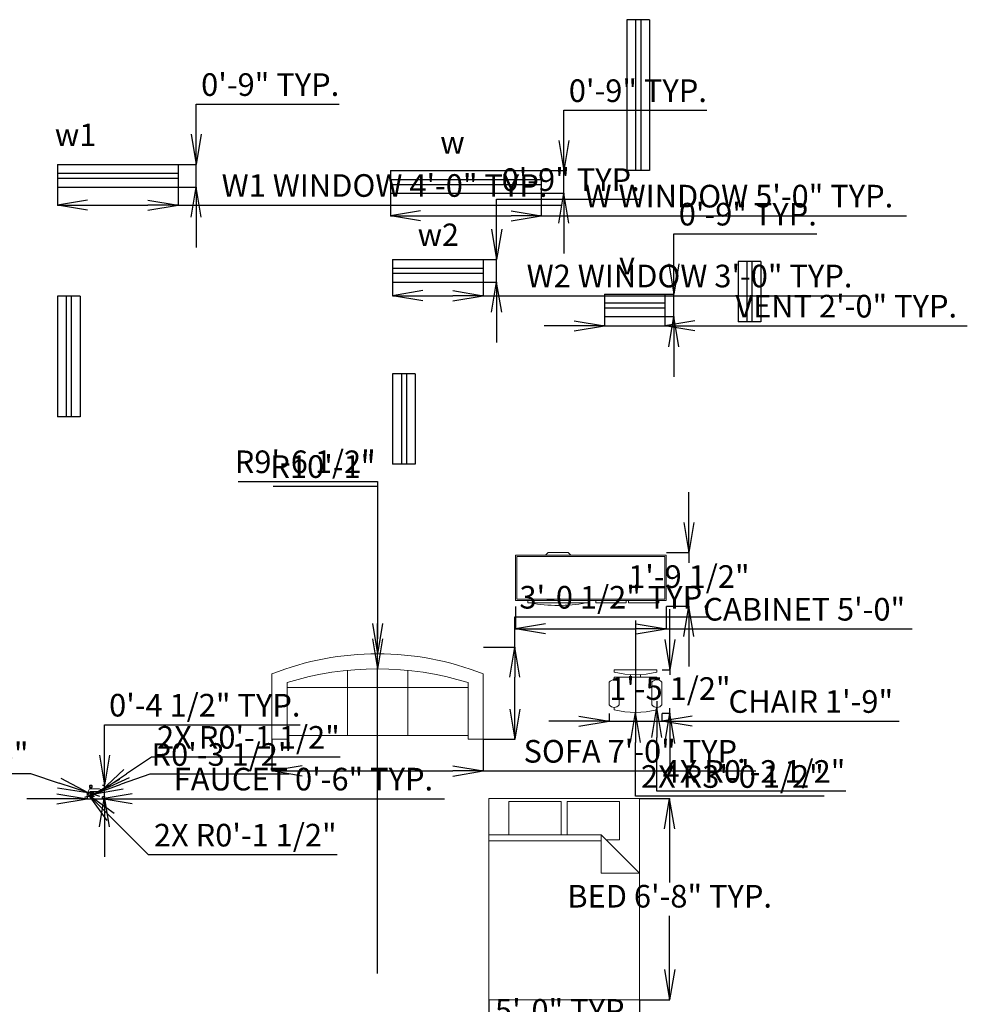
# Model space of a CAD drawing. Units: inches. Extents: x 1856 to 3350, y 1624 to 2224.
# Tile 7 of 7: x 2954 to 3331, y 1823 to 2214. Entities that reach past the tile are written whole.
import ezdxf

# ---------------------------------------------------------------- set-up
doc = ezdxf.new("R2010")
doc.units = ezdxf.units.IN
for name, color, linetype, lineweight in [('A-ANNO-DIMS', 2, 'Continuous', 18), ('A-ANNO-TEXT', 7, 'Continuous', 18), ('A-FLOR-FIXT', 3, 'Continuous', 18), ('A-FURN', 3, 'Continuous', 18), ('ventilator', 6, 'Continuous', 25), ('window', 4, 'Continuous', 25)]:
    doc.layers.add(name, color=color, linetype=linetype, lineweight=lineweight)
doc.styles.get("Standard").update_dxf_attribs({"font": 'arial.ttf'})
doc.dimstyles.new('ISO-25', dxfattribs={"dimtxt": 9, "dimasz": 12, "dimexe": 0.125, "dimexo": 0.125, "dimgap": 2, "dimtad": 1, "dimtih": 1, "dimtoh": 1, "dimdec": 1, "dimzin": 11, "dimlunit": 4, "dimtxsty": 'Standard', "dimblk": 'OPEN', "dimcen": -0.125, "dimadec": 0, "dimazin": 0, "dimtfac": 1, "dimtdec": 1, "dimtmove": 0, "dimatfit": 3, "dimfxl": 1, "dimarcsym": 0})

# ---------------------------------------------------------------- blocks, each defined once
blk = doc.blocks.new('Chair - Desk')
for p, q in [((-8.5, 0), (-8.5, -1)), ((-8.5, 0), (8.5, 0)), ((8.5, 0), (8.5, -1)), ((-8.5, -3), (-8.5, -4)), ((-8.5, -3), (8.5, -3)), ((-2, -3), (-2, -1.9355)), ((2, -1.9576), (2, -3)), ((8.5, -3), (8.5, -4)), ((-10.5, -5), (-10.5, -14)), ((-6.5, -14), (-6.5, -5)), ((6.5, -5), (6.5, -14)), ((10.5, -14), (10.5, -5)), ((-8.5, -15), (-8.5, -16)), ((8.5, -15), (8.5, -16))]:
    blk.add_line(p, q)
for centre, radius, start, end in [((0, 34.625), 36.625, 256.5803, 283.4197), ((-8.5, -6.5), 2.5, 36.8699, 143.1301), ((8.5, -6.5), 2.5, 36.8699, 143.1301), ((-8.5, -12.5), 2.5, 216.8699, 323.1301), ((8.5, -12.5), 2.5, 216.8699, 323.1301), ((0, 19.625), 36.625, 256.5803, 283.4197)]:
    blk.add_arc(centre, radius, start, end)
blk = doc.blocks.new('Bed - Queen')
for p, q in [((0, -80.00003), (0, 0)), ((0, 0), (59.99999, 0)), ((59.99999, 0), (59.99999, -80.00003)), ((7.99999, -1.2), (28.79998, -1.2)), ((7.99999, -14.4), (7.99999, -1.2)), ((28.79998, -1.2), (28.79998, -14.4)), ((31.19999, -1.2), (51.99999, -1.2)), ((31.19999, -14.4), (31.19999, -1.2)), ((51.99999, -1.2), (51.99999, -16.4)), ((0, -14.4), (44.8, -14.4)), ((59.99999, -29.6), (44.8, -14.4)), ((44.8, -14.4), (44.8, -29.6)), ((44.8, -16.8), (0, -16.8)), ((51.99999, -16.4), (46.79936, -16.4)), ((44.8, -29.6), (59.99999, -29.6)), ((59.99999, -80.00003), (0, -80.00003))]:
    blk.add_line(p, q)
blk = doc.blocks.new('Entertainment Center')
for p, q in [((-4, 0), (-5, -1)), ((4, 0), (-4, 0)), ((5, -1), (4, 0)), ((-17, -19), (-17, -1)), ((-17, -1), (43, -1)), ((-16.5, -18.5), (-16.5, -1.5)), ((-16.5, -1.5), (42.5, -1.5)), ((42.5, -1.5), (42.5, -18.5)), ((43, -1), (43, -19)), ((43, -19), (-17, -19)), ((42.5, -18.5), (-16.5, -18.5)), ((-12, -20), (-12, -19)), ((12, -19), (12, -20)), ((15, -20), (15, -19)), ((27, -19), (27, -20)), ((28, -20), (28, -19)), ((40, -19), (40, -20)), ((12, -20), (-12, -20)), ((27, -20), (15, -20)), ((40, -20), (28, -20))]:
    blk.add_line(p, q)
blk.add_arc((0, 40), 61, 259.6111, 280.3889)
blk = doc.blocks.new('Sofa - Roundback 7 ft.')
for p, q in [((-12.00002, -32.4421), (-12.00003, -6.5971)), ((11.99997, -32.4421), (11.99998, -6.5971)), ((-36.000027, -34), (-36.000027, -11.4696)), ((35.99998, -34), (35.99998, -11.4696)), ((-35.999844, -13.3819), (35.9998, -13.3819)), ((-36.000027, -32.4421), (35.99998, -32.4421))]:
    blk.add_line(p, q)
for points in [[(-36.000027, -34), (-42.000027, -34), (-42.000027, -8)], [(41.99998, -8), (41.99998, -34), (35.99998, -34)]]:
    blk.add_lwpolyline(points)
for centre, radius, start, end in [((0, -114.25), 114.25, 68.43141, 111.5686), ((-0.00001, -127.1968), 121.1968, 72.72033, 107.2797)]:
    blk.add_arc(centre, radius, start, end)
blk = doc.blocks.new('Faucet - Bathroom side')
for p, q in [((-0.625, 4.25), (0.375, 4.25)), ((-1.625, 0), (-1.375, 0)), ((-1.375, 0), (1.375, 0)), ((-0.88366, 0.25), (0.88424, 0.25)), ((0.375, 3.75), (-0.625, 3.75)), ((-0.625, 3), (3.375, 3)), ((-0.375, 1.625), (-0.625, 1.625)), ((-0.375, 1.375), (-0.625, 1.375)), ((0.48078, 0.75), (-0.47286, 0.75)), ((-0.375, 3), (-0.375, 3.5)), ((0.125, 3.5), (0.125, 3)), ((2.875, 2), (0.375, 2)), ((0.375, 1.625), (0.625, 1.625)), ((0.375, 1.375), (0.625, 1.375)), ((4.375, 1.5), (3.375, 1.5))]:
    blk.add_line(p, q)
for points in [[(-0.625, 3.75), (-0.625, 4.25)], [(-0.375, 4.5), (0.125, 4.5)], [(0.375, 4.25), (0.375, 3.75)], [(0.125, 3.5), (-0.375, 3.5)]]:
    blk.add_lwpolyline(points)
blk.add_lwpolyline([(-0.375, 1), (-0.375, 2), (0.375, 2), (0.375, 1)], close=True)
for centre in [(-0.875, 1.5), (0, 1.5), (0.875, 1.5)]:
    blk.add_circle(centre, 0.27951)
for centre, radius, start, end in [((-0.38253, 4.2575), 0.24259, 88.22243, 181.7776), ((0.13252, 4.2575), 0.24259, 358.2224, 91.77757), ((3.45929, -0.0281), 5.08436, 143.4467, 179.6834), ((-1.75, 1.375), 1.42522, 285.2551, 344.7449), ((-0.38253, 3.7424), 0.24259, 178.2224, 271.7776), ((0.13252, 3.7424), 0.24259, 268.2224, 1.777565), ((1.75, 1.375), 1.42522, 195.2551, 254.7449), ((-2.49562, -0.286), 3.38273, 9.709485, 29.48735), ((2.96867, 1.5936), 0.41699, 347.0192, 102.9808), ((2.70708, 1.4714), 1.66816, 0.9827695, 66.39737)]:
    blk.add_arc(centre, radius, start, end)
blk = doc.blocks.new('WIN-48')
for p, q in [((0, 9), (48, 9)), ((0, 9), (0, 0)), ((48, 9), (48, 0)), ((0, 5.5), (48, 5.5)), ((0, 3.5), (48, 3.5)), ((0, 0), (48, 0))]:
    blk.add_line(p, q)
blk = doc.blocks.new('WIN-60')
for p, q in [((0, 9), (60, 9)), ((0, 9), (0, 0)), ((60, 9), (60, 0)), ((0, 5.5), (60, 5.5)), ((0, 3.5), (60, 3.5)), ((0, 0), (60, 0))]:
    blk.add_line(p, q)
blk = doc.blocks.new('WIN-36')
for p, q in [((0, 9), (36, 9)), ((0, 9), (0, 0)), ((36, 9), (36, 0)), ((0, 5.5), (36, 5.5)), ((0, 3.5), (36, 3.5)), ((0, 0), (36, 0))]:
    blk.add_line(p, q)
blk = doc.blocks.new('VENT-24')
for p, q in [((0, 9), (24, 9)), ((0, 9), (0, 0)), ((24, 9), (24, 0)), ((0, 5.5), (24, 5.5)), ((0, 3.5), (24, 3.5)), ((0, 0), (24, 0))]:
    blk.add_line(p, q)
blk = doc.blocks.new('_Open')
at = {"color": 0, "linetype": 'ByBlock', "lineweight": -2}
for p, q in [((-1, 0.167), (0, 0)), ((-1, -0.167), (0, 0)), ((0, 0), (-1, 0))]:
    blk.add_line(p, q, dxfattribs=at)
blk = doc.blocks.new('*D26')
at = {"layer": 'A-ANNO-DIMS', "color": 0, "lineweight": -2, "transparency": 16777216}
for p, q in [((2969.28, 2147.66), (2969.28, 2140.46)), ((3017.28, 2147.66), (3017.28, 2140.46)), ((2981.28, 2140.58), (3005.28, 2140.58)), ((3017.28, 2140.58), (3169.52, 2140.58))]:
    blk.add_line(p, q, dxfattribs=at)
at = {"layer": 'Defpoints', "color": 0, "transparency": 16777216}
for p in [(2969.28, 2147.78), (3017.28, 2147.78), (3017.28, 2140.58)]:
    blk.add_point(p, dxfattribs=at)
at = {"layer": 'A-ANNO-DIMS', "color": 0, "lineweight": -2, "transparency": 16777216, "xscale": 12, "yscale": 12, "zscale": 12, "rotation": 180}
blk.add_blockref('_Open', (2969.28, 2140.58), dxfattribs=at)
at = {"layer": 'A-ANNO-DIMS', "color": 0, "lineweight": -2, "transparency": 16777216, "xscale": 12, "yscale": 12, "zscale": 12}
blk.add_blockref('_Open', (3017.28, 2140.58), dxfattribs=at)
at = {"layer": 'A-ANNO-DIMS', "color": 0, "transparency": 16777216, "insert": (3099.4, 2147.24), "char_height": 9, "attachment_point": 5}
blk.add_mtext('W1 WINDOW 4\'-0" TYP.', dxfattribs=at)
blk = doc.blocks.new('*D27')
at = {"layer": 'A-ANNO-DIMS', "color": 0, "lineweight": -2, "transparency": 16777216}
for p, q in [((3024.48, 2168.78), (3024.48, 2180.78)), ((3024.48, 2180.78), (3081.34, 2180.78)), ((3017.41, 2156.78), (3024.61, 2156.78)), ((3024.48, 2147.78), (3024.48, 2156.78)), ((3017.41, 2147.78), (3024.61, 2147.78)), ((3024.48, 2135.78), (3024.48, 2123.78))]:
    blk.add_line(p, q, dxfattribs=at)
at = {"layer": 'Defpoints', "color": 0, "transparency": 16777216}
for p in [(3017.28, 2156.78), (3024.48, 2156.78), (3017.28, 2147.78)]:
    blk.add_point(p, dxfattribs=at)
at = {"layer": 'A-ANNO-DIMS', "color": 0, "lineweight": -2, "transparency": 16777216, "xscale": 12, "yscale": 12, "zscale": 12}
for p, rotation in [((3024.48, 2156.78), 270), ((3024.48, 2147.78), 90)]:
    blk.add_blockref('_Open', p, dxfattribs=dict(at, rotation=rotation))
at = {"layer": 'A-ANNO-DIMS', "color": 0, "transparency": 16777216, "insert": (3053.91, 2187.38), "char_height": 9, "attachment_point": 5}
blk.add_mtext('0\'-9" TYP.', dxfattribs=at)
blk = doc.blocks.new('*D28')
at = {"layer": 'A-ANNO-DIMS', "color": 0, "lineweight": -2, "transparency": 16777216}
for p, q in [((3101.75, 2145.23), (3101.75, 2136.23)), ((3161.75, 2145.23), (3161.75, 2136.23)), ((3113.75, 2136.36), (3149.75, 2136.36)), ((3161.75, 2136.36), (3307, 2136.36))]:
    blk.add_line(p, q, dxfattribs=at)
at = {"layer": 'Defpoints', "color": 0, "transparency": 16777216}
for p in [(3101.75, 2145.36), (3161.75, 2145.36), (3161.75, 2136.36)]:
    blk.add_point(p, dxfattribs=at)
at = {"layer": 'A-ANNO-DIMS', "color": 0, "lineweight": -2, "transparency": 16777216, "xscale": 12, "yscale": 12, "zscale": 12, "rotation": 180}
blk.add_blockref('_Open', (3101.75, 2136.36), dxfattribs=at)
at = {"layer": 'A-ANNO-DIMS', "color": 0, "lineweight": -2, "transparency": 16777216, "xscale": 12, "yscale": 12, "zscale": 12}
blk.add_blockref('_Open', (3161.75, 2136.36), dxfattribs=at)
at = {"layer": 'A-ANNO-DIMS', "color": 0, "transparency": 16777216, "insert": (3240.37, 2143.01), "char_height": 9, "attachment_point": 5}
blk.add_mtext('W WINDOW 5\'-0" TYP.', dxfattribs=at)
blk = doc.blocks.new('*D29')
at = {"layer": 'A-ANNO-DIMS', "color": 0, "lineweight": -2, "transparency": 16777216}
for p, q in [((3170.75, 2166.36), (3170.75, 2178.36)), ((3170.75, 2178.36), (3227.61, 2178.36)), ((3161.87, 2154.36), (3170.87, 2154.36)), ((3170.75, 2145.36), (3170.75, 2154.36)), ((3161.87, 2145.36), (3170.87, 2145.36)), ((3170.75, 2133.36), (3170.75, 2121.36))]:
    blk.add_line(p, q, dxfattribs=at)
at = {"layer": 'Defpoints', "color": 0, "transparency": 16777216}
for p in [(3161.75, 2154.36), (3170.75, 2154.36), (3161.75, 2145.36)]:
    blk.add_point(p, dxfattribs=at)
at = {"layer": 'A-ANNO-DIMS', "color": 0, "lineweight": -2, "transparency": 16777216, "xscale": 12, "yscale": 12, "zscale": 12}
for p, rotation in [((3170.75, 2154.36), 270), ((3170.75, 2145.36), 90)]:
    blk.add_blockref('_Open', p, dxfattribs=dict(at, rotation=rotation))
at = {"layer": 'A-ANNO-DIMS', "color": 0, "transparency": 16777216, "insert": (3200.18, 2184.95), "char_height": 9, "attachment_point": 5}
blk.add_mtext('0\'-9" TYP.', dxfattribs=at)
blk = doc.blocks.new('*D30')
at = {"layer": 'A-ANNO-DIMS', "color": 0, "lineweight": -2, "transparency": 16777216}
for p, q in [((3102.61, 2109.86), (3102.61, 2104.46)), ((3138.61, 2109.86), (3138.61, 2104.46)), ((3114.61, 2104.58), (3126.61, 2104.58)), ((3138.61, 2104.58), (3290.85, 2104.58))]:
    blk.add_line(p, q, dxfattribs=at)
at = {"layer": 'Defpoints', "color": 0, "transparency": 16777216}
for p in [(3102.61, 2109.98), (3138.61, 2109.98), (3138.61, 2104.58)]:
    blk.add_point(p, dxfattribs=at)
at = {"layer": 'A-ANNO-DIMS', "color": 0, "lineweight": -2, "transparency": 16777216, "xscale": 12, "yscale": 12, "zscale": 12, "rotation": 180}
blk.add_blockref('_Open', (3102.61, 2104.58), dxfattribs=at)
at = {"layer": 'A-ANNO-DIMS', "color": 0, "lineweight": -2, "transparency": 16777216, "xscale": 12, "yscale": 12, "zscale": 12}
blk.add_blockref('_Open', (3138.61, 2104.58), dxfattribs=at)
at = {"layer": 'A-ANNO-DIMS', "color": 0, "transparency": 16777216, "insert": (3220.73, 2111.24), "char_height": 9, "attachment_point": 5}
blk.add_mtext('W2 WINDOW 3\'-0" TYP.', dxfattribs=at)
blk = doc.blocks.new('*D31')
at = {"layer": 'A-ANNO-DIMS', "color": 0, "lineweight": -2, "transparency": 16777216}
for p, q in [((3144.01, 2130.98), (3144.01, 2142.98)), ((3144.01, 2142.98), (3200.87, 2142.98)), ((3138.74, 2118.98), (3144.14, 2118.98)), ((3144.01, 2109.98), (3144.01, 2118.98)), ((3138.74, 2109.98), (3144.14, 2109.98)), ((3144.01, 2097.98), (3144.01, 2085.98))]:
    blk.add_line(p, q, dxfattribs=at)
at = {"layer": 'Defpoints', "color": 0, "transparency": 16777216}
for p in [(3138.61, 2118.98), (3144.01, 2118.98), (3138.61, 2109.98)]:
    blk.add_point(p, dxfattribs=at)
at = {"layer": 'A-ANNO-DIMS', "color": 0, "lineweight": -2, "transparency": 16777216, "xscale": 12, "yscale": 12, "zscale": 12}
for p, rotation in [((3144.01, 2118.98), 270), ((3144.01, 2109.98), 90)]:
    blk.add_blockref('_Open', p, dxfattribs=dict(at, rotation=rotation))
at = {"layer": 'A-ANNO-DIMS', "color": 0, "transparency": 16777216, "insert": (3173.44, 2149.58), "char_height": 9, "attachment_point": 5}
blk.add_mtext('0\'-9" TYP.', dxfattribs=at)
blk = doc.blocks.new('*D32')
at = {"layer": 'A-ANNO-DIMS', "color": 0, "lineweight": -2, "transparency": 16777216}
for p, q in [((3186.89, 2096.12), (3186.89, 2092.52)), ((3210.89, 2096.12), (3210.89, 2092.52)), ((3174.89, 2092.64), (3162.89, 2092.64)), ((3186.89, 2092.64), (3210.89, 2092.64)), ((3222.89, 2092.64), (3331.25, 2092.64))]:
    blk.add_line(p, q, dxfattribs=at)
at = {"layer": 'Defpoints', "color": 0, "transparency": 16777216}
for p in [(3186.89, 2096.24), (3210.89, 2096.24), (3210.89, 2092.64)]:
    blk.add_point(p, dxfattribs=at)
at = {"layer": 'A-ANNO-DIMS', "color": 0, "lineweight": -2, "transparency": 16777216, "xscale": 12, "yscale": 12, "zscale": 12}
blk.add_blockref('_Open', (3186.89, 2092.64), dxfattribs=at)
at = {"layer": 'A-ANNO-DIMS', "color": 0, "lineweight": -2, "transparency": 16777216, "xscale": 12, "yscale": 12, "zscale": 12, "rotation": 180}
blk.add_blockref('_Open', (3210.89, 2092.64), dxfattribs=at)
at = {"layer": 'A-ANNO-DIMS', "color": 0, "transparency": 16777216, "insert": (3283.07, 2099.24), "char_height": 9, "attachment_point": 5}
blk.add_mtext('VENT 2\'-0" TYP.', dxfattribs=at)
blk = doc.blocks.new('*D33')
at = {"layer": 'A-ANNO-DIMS', "color": 0, "lineweight": -2, "transparency": 16777216}
for p, q in [((3214.49, 2117.24), (3214.49, 2129.24)), ((3214.49, 2129.24), (3271.35, 2129.24)), ((3211.02, 2105.24), (3214.62, 2105.24)), ((3214.49, 2096.24), (3214.49, 2105.24)), ((3211.02, 2096.24), (3214.62, 2096.24)), ((3214.49, 2084.24), (3214.49, 2072.24))]:
    blk.add_line(p, q, dxfattribs=at)
at = {"layer": 'Defpoints', "color": 0, "transparency": 16777216}
for p in [(3210.89, 2105.24), (3214.49, 2105.24), (3210.89, 2096.24)]:
    blk.add_point(p, dxfattribs=at)
at = {"layer": 'A-ANNO-DIMS', "color": 0, "lineweight": -2, "transparency": 16777216, "xscale": 12, "yscale": 12, "zscale": 12}
for p, rotation in [((3214.49, 2105.24), 270), ((3214.49, 2096.24), 90)]:
    blk.add_blockref('_Open', p, dxfattribs=dict(at, rotation=rotation))
at = {"layer": 'A-ANNO-DIMS', "color": 0, "transparency": 16777216, "insert": (3243.92, 2135.84), "char_height": 9, "attachment_point": 5}
blk.add_mtext('0\'-9" TYP.', dxfattribs=at)
blk = doc.blocks.new('*D34')
at = {"layer": 'A-ANNO-DIMS', "color": 0, "lineweight": -2, "transparency": 16777216}
for p, q in [((3200.96, 1904.55), (3212.96, 1904.55)), ((3212.83, 1892.55), (3212.83, 1871.14)), ((3212.83, 1836.55), (3212.83, 1857.95)), ((3200.96, 1824.55), (3212.96, 1824.55))]:
    blk.add_line(p, q, dxfattribs=at)
at = {"layer": 'Defpoints', "color": 0, "transparency": 16777216}
for p in [(3200.83, 1904.55), (3212.83, 1904.55), (3200.83, 1824.55)]:
    blk.add_point(p, dxfattribs=at)
at = {"layer": 'A-ANNO-DIMS', "color": 0, "lineweight": -2, "transparency": 16777216, "xscale": 12, "yscale": 12, "zscale": 12}
for p, rotation in [((3212.83, 1904.55), 90), ((3212.83, 1824.55), 270)]:
    blk.add_blockref('_Open', p, dxfattribs=dict(at, rotation=rotation))
at = {"layer": 'A-ANNO-DIMS', "color": 0, "transparency": 16777216, "insert": (3212.83, 1864.55), "char_height": 9, "attachment_point": 5}
blk.add_mtext('BED 6\'-8" TYP.', dxfattribs=at)
blk = doc.blocks.new('*D35')
at = {"layer": 'A-ANNO-DIMS', "color": 0, "lineweight": -2, "transparency": 16777216}
for p, q in [((3140.83, 1824.42), (3140.83, 1812.42)), ((3200.83, 1824.42), (3200.83, 1812.42)), ((3152.83, 1812.55), (3188.83, 1812.55))]:
    blk.add_line(p, q, dxfattribs=at)
at = {"layer": 'Defpoints', "color": 0, "transparency": 16777216}
for p in [(3140.83, 1824.55), (3200.83, 1824.55), (3200.83, 1812.55)]:
    blk.add_point(p, dxfattribs=at)
at = {"layer": 'A-ANNO-DIMS', "color": 0, "lineweight": -2, "transparency": 16777216, "xscale": 12, "yscale": 12, "zscale": 12, "rotation": 180}
blk.add_blockref('_Open', (3140.83, 1812.55), dxfattribs=at)
at = {"layer": 'A-ANNO-DIMS', "color": 0, "lineweight": -2, "transparency": 16777216, "xscale": 12, "yscale": 12, "zscale": 12}
blk.add_blockref('_Open', (3200.83, 1812.55), dxfattribs=at)
at = {"layer": 'A-ANNO-DIMS', "color": 0, "transparency": 16777216, "insert": (3170.83, 1819.14), "char_height": 9, "attachment_point": 5}
blk.add_mtext('5\'-0" TYP.', dxfattribs=at)
blk = doc.blocks.new('*D36')
at = {"layer": 'A-ANNO-DIMS', "color": 0, "lineweight": -2, "transparency": 16777216}
for p, q in [((3151.47, 1980.91), (3151.47, 1971.91)), ((3211.47, 1980.91), (3211.47, 1971.91)), ((3163.47, 1972.04), (3199.47, 1972.04)), ((3211.47, 1972.04), (3309.27, 1972.04))]:
    blk.add_line(p, q, dxfattribs=at)
at = {"layer": 'Defpoints', "color": 0, "transparency": 16777216}
for p in [(3151.47, 1981.04), (3211.47, 1981.04), (3211.47, 1972.04)]:
    blk.add_point(p, dxfattribs=at)
at = {"layer": 'A-ANNO-DIMS', "color": 0, "lineweight": -2, "transparency": 16777216, "xscale": 12, "yscale": 12, "zscale": 12, "rotation": 180}
blk.add_blockref('_Open', (3151.47, 1972.04), dxfattribs=at)
at = {"layer": 'A-ANNO-DIMS', "color": 0, "lineweight": -2, "transparency": 16777216, "xscale": 12, "yscale": 12, "zscale": 12}
blk.add_blockref('_Open', (3211.47, 1972.04), dxfattribs=at)
at = {"layer": 'A-ANNO-DIMS', "color": 0, "transparency": 16777216, "insert": (3266.37, 1978.69), "char_height": 9, "attachment_point": 5}
blk.add_mtext('CABINET 5\'-0"', dxfattribs=at)
blk = doc.blocks.new('*D37')
at = {"layer": 'A-ANNO-DIMS', "color": 0, "lineweight": -2, "transparency": 16777216}
for p, q in [((3220.47, 2014.37), (3220.47, 2026.37)), ((3211.59, 2002.37), (3220.59, 2002.37)), ((3220.47, 2002.37), (3220.47, 1998.36)), ((3220.47, 1981.04), (3220.47, 1985.05)), ((3211.59, 1981.04), (3220.59, 1981.04)), ((3220.47, 1969.04), (3220.47, 1957.04))]:
    blk.add_line(p, q, dxfattribs=at)
at = {"layer": 'Defpoints', "color": 0, "transparency": 16777216}
for p in [(3211.47, 2002.37), (3220.47, 2002.37), (3211.47, 1981.04)]:
    blk.add_point(p, dxfattribs=at)
at = {"layer": 'A-ANNO-DIMS', "color": 0, "lineweight": -2, "transparency": 16777216, "xscale": 12, "yscale": 12, "zscale": 12}
for p, rotation in [((3220.47, 2002.37), 270), ((3220.47, 1981.04), 90)]:
    blk.add_blockref('_Open', p, dxfattribs=dict(at, rotation=rotation))
at = {"layer": 'A-ANNO-DIMS', "color": 0, "transparency": 16777216, "insert": (3220.47, 1991.7), "char_height": 9, "attachment_point": 5}
blk.add_mtext('1\'-9 1/2"', dxfattribs=at)
blk = doc.blocks.new('*D38')
at = {"layer": 'A-ANNO-DIMS', "color": 0, "lineweight": -2, "transparency": 16777216}
for p, q in [((3176.76, 1935.34), (3164.76, 1935.34)), ((3188.76, 1938.37), (3188.76, 1935.22)), ((3188.76, 1935.34), (3209.76, 1935.34)), ((3209.76, 1938.37), (3209.76, 1935.22)), ((3221.76, 1935.34), (3304.19, 1935.34))]:
    blk.add_line(p, q, dxfattribs=at)
at = {"layer": 'Defpoints', "color": 0, "transparency": 16777216}
for p in [(3188.76, 1938.49), (3209.76, 1938.49), (3209.76, 1935.34)]:
    blk.add_point(p, dxfattribs=at)
at = {"layer": 'A-ANNO-DIMS', "color": 0, "lineweight": -2, "transparency": 16777216, "xscale": 12, "yscale": 12, "zscale": 12}
blk.add_blockref('_Open', (3188.76, 1935.34), dxfattribs=at)
at = {"layer": 'A-ANNO-DIMS', "color": 0, "lineweight": -2, "transparency": 16777216, "xscale": 12, "yscale": 12, "zscale": 12, "rotation": 180}
blk.add_blockref('_Open', (3209.76, 1935.34), dxfattribs=at)
at = {"layer": 'A-ANNO-DIMS', "color": 0, "transparency": 16777216, "insert": (3268.98, 1942), "char_height": 9, "attachment_point": 5}
blk.add_mtext('CHAIR 1\'-9"', dxfattribs=at)
blk = doc.blocks.new('*D39')
at = {"layer": 'A-ANNO-DIMS', "color": 0, "lineweight": -2, "transparency": 16777216}
for p, q in [((3212.91, 1967.83), (3212.91, 1979.83)), ((3209.89, 1955.83), (3213.04, 1955.83)), ((3212.91, 1955.83), (3212.91, 1953.81)), ((3212.91, 1938.49), (3212.91, 1940.51)), ((3209.89, 1938.49), (3213.04, 1938.49)), ((3212.91, 1926.49), (3212.91, 1914.49))]:
    blk.add_line(p, q, dxfattribs=at)
at = {"layer": 'Defpoints', "color": 0, "transparency": 16777216}
for p in [(3209.76, 1955.83), (3212.91, 1955.83), (3209.76, 1938.49)]:
    blk.add_point(p, dxfattribs=at)
at = {"layer": 'A-ANNO-DIMS', "color": 0, "lineweight": -2, "transparency": 16777216, "xscale": 12, "yscale": 12, "zscale": 12}
for p, rotation in [((3212.91, 1955.83), 270), ((3212.91, 1938.49), 90)]:
    blk.add_blockref('_Open', p, dxfattribs=dict(at, rotation=rotation))
at = {"layer": 'A-ANNO-DIMS', "color": 0, "transparency": 16777216, "insert": (3212.91, 1947.16), "char_height": 9, "attachment_point": 5}
blk.add_mtext('1\'-5 1/2"', dxfattribs=at)
blk = doc.blocks.new('*D40')
at = {"layer": 'A-ANNO-DIMS', "color": 0, "lineweight": -2, "transparency": 16777216}
for p, q in [((3054.62, 1928.01), (3054.62, 1915.41)), ((3138.62, 1928.01), (3138.62, 1915.41)), ((3066.62, 1915.54), (3126.62, 1915.54)), ((3138.62, 1915.54), (3247.16, 1915.54))]:
    blk.add_line(p, q, dxfattribs=at)
at = {"layer": 'Defpoints', "color": 0, "transparency": 16777216}
for p in [(3054.62, 1928.14), (3138.62, 1928.14), (3138.62, 1915.54)]:
    blk.add_point(p, dxfattribs=at)
at = {"layer": 'A-ANNO-DIMS', "color": 0, "lineweight": -2, "transparency": 16777216, "xscale": 12, "yscale": 12, "zscale": 12, "rotation": 180}
blk.add_blockref('_Open', (3054.62, 1915.54), dxfattribs=at)
at = {"layer": 'A-ANNO-DIMS', "color": 0, "lineweight": -2, "transparency": 16777216, "xscale": 12, "yscale": 12, "zscale": 12}
blk.add_blockref('_Open', (3138.62, 1915.54), dxfattribs=at)
at = {"layer": 'A-ANNO-DIMS', "color": 0, "transparency": 16777216, "insert": (3198.89, 1922.19), "char_height": 9, "attachment_point": 5}
blk.add_mtext('SOFA 7\'-0" TYP.', dxfattribs=at)
blk = doc.blocks.new('*D41')
at = {"layer": 'A-ANNO-DIMS', "color": 0, "lineweight": -2, "transparency": 16777216}
for p, q in [((3151.22, 1964.8), (3151.22, 1976.8)), ((3151.22, 1976.8), (3229.04, 1976.8)), ((3138.74, 1964.8), (3151.34, 1964.8)), ((3151.22, 1940.14), (3151.22, 1952.8)), ((3138.74, 1928.14), (3151.34, 1928.14))]:
    blk.add_line(p, q, dxfattribs=at)
at = {"layer": 'Defpoints', "color": 0, "transparency": 16777216}
for p in [(3138.62, 1964.8), (3151.22, 1964.8), (3138.62, 1928.14)]:
    blk.add_point(p, dxfattribs=at)
at = {"layer": 'A-ANNO-DIMS', "color": 0, "lineweight": -2, "transparency": 16777216, "xscale": 12, "yscale": 12, "zscale": 12}
for p, rotation in [((3151.22, 1964.8), 90), ((3151.22, 1928.14), 270)]:
    blk.add_blockref('_Open', p, dxfattribs=dict(at, rotation=rotation))
at = {"layer": 'A-ANNO-DIMS', "color": 0, "transparency": 16777216, "insert": (3191.13, 1983.46), "char_height": 9, "attachment_point": 5}
blk.add_mtext('3\'-0 1/2" TYP.', dxfattribs=at)
blk = doc.blocks.new('*D56')
at = {"layer": 'A-ANNO-DIMS', "color": 0, "lineweight": -2, "transparency": 16777216}
for p, q in [((2969.06, 1904.47), (2957.06, 1904.47)), ((2981.06, 1905.25), (2981.06, 1904.35)), ((2981.06, 1904.47), (2987.06, 1904.47)), ((2987.06, 1905.25), (2987.06, 1904.35)), ((2999.06, 1904.47), (3123.2, 1904.47))]:
    blk.add_line(p, q, dxfattribs=at)
at = {"layer": 'Defpoints', "color": 0, "transparency": 16777216}
for p in [(2981.06, 1905.37), (2987.06, 1905.37), (2987.06, 1904.47)]:
    blk.add_point(p, dxfattribs=at)
at = {"layer": 'A-ANNO-DIMS', "color": 0, "lineweight": -2, "transparency": 16777216, "xscale": 12, "yscale": 12, "zscale": 12}
blk.add_blockref('_Open', (2981.06, 1904.47), dxfattribs=at)
at = {"layer": 'A-ANNO-DIMS', "color": 0, "lineweight": -2, "transparency": 16777216, "xscale": 12, "yscale": 12, "zscale": 12, "rotation": 180}
blk.add_blockref('_Open', (2987.06, 1904.47), dxfattribs=at)
at = {"layer": 'A-ANNO-DIMS', "color": 0, "transparency": 16777216, "insert": (3067.13, 1911.13), "char_height": 9, "attachment_point": 5}
blk.add_mtext('FAUCET 0\'-6" TYP.', dxfattribs=at)
blk = doc.blocks.new('*D57')
at = {"layer": 'A-ANNO-DIMS', "color": 0, "lineweight": -2, "transparency": 16777216}
for p, q in [((2987.96, 1921.87), (2987.96, 1933.87)), ((2987.96, 1933.87), (3065.79, 1933.87)), ((2987.19, 1909.87), (2988.09, 1909.87)), ((2987.96, 1905.37), (2987.96, 1909.87)), ((2987.19, 1905.37), (2988.09, 1905.37)), ((2987.96, 1893.37), (2987.96, 1881.37))]:
    blk.add_line(p, q, dxfattribs=at)
at = {"layer": 'Defpoints', "color": 0, "transparency": 16777216}
for p in [(2987.06, 1909.87), (2987.96, 1909.87), (2987.06, 1905.37)]:
    blk.add_point(p, dxfattribs=at)
at = {"layer": 'A-ANNO-DIMS', "color": 0, "lineweight": -2, "transparency": 16777216, "xscale": 12, "yscale": 12, "zscale": 12}
for p, rotation in [((2987.96, 1909.87), 270), ((2987.96, 1905.37), 90)]:
    blk.add_blockref('_Open', p, dxfattribs=dict(at, rotation=rotation))
at = {"layer": 'A-ANNO-DIMS', "color": 0, "transparency": 16777216, "insert": (3027.88, 1940.53), "char_height": 9, "attachment_point": 5}
blk.add_mtext('0\'-4 1/2" TYP.', dxfattribs=at)
blk = doc.blocks.new('*D93')
at = {"layer": 'A-ANNO-DIMS', "color": 0, "lineweight": -2, "transparency": 16777216}
for p, q in [((3055.09, 2028.85), (3096.62, 2028.85)), ((3096.62, 2028.85), (3096.62, 1968.14)), ((3096.62, 1834.94), (3096.62, 1956.14))]:
    blk.add_line(p, q, dxfattribs=at)
at = {"layer": 'Defpoints', "color": 0, "transparency": 16777216}
for p in [(3096.62, 1956.14), (3096.62, 1834.94)]:
    blk.add_point(p, dxfattribs=at)
at = {"layer": 'A-ANNO-DIMS', "color": 0, "lineweight": -2, "transparency": 16777216, "xscale": 12, "yscale": 12, "zscale": 12, "rotation": 270.0002075372221}
blk.add_blockref('_Open', (3096.62, 1956.14), dxfattribs=at)
at = {"layer": 'A-ANNO-DIMS', "color": 0, "transparency": 16777216, "insert": (3074.85, 2035.45), "char_height": 9, "attachment_point": 5}
blk.add_mtext('R10\'-1"', dxfattribs=at)
blk = doc.blocks.new('*D94')
at = {"layer": 'A-ANNO-DIMS', "color": 0, "lineweight": -2, "transparency": 16777216}
for p, q in [((3041.11, 2030.69), (3096.62, 2030.69)), ((3096.62, 2030.69), (3096.62, 1974.14)), ((3096.62, 1847.89), (3096.62, 1962.14))]:
    blk.add_line(p, q, dxfattribs=at)
at = {"layer": 'Defpoints', "color": 0, "transparency": 16777216}
for p in [(3096.62, 1962.14), (3096.62, 1847.89)]:
    blk.add_point(p, dxfattribs=at)
at = {"layer": 'A-ANNO-DIMS', "color": 0, "lineweight": -2, "transparency": 16777216, "xscale": 12, "yscale": 12, "zscale": 12, "rotation": 270.0002251711596}
blk.add_blockref('_Open', (3096.62, 1962.14), dxfattribs=at)
at = {"layer": 'A-ANNO-DIMS', "color": 0, "transparency": 16777216, "insert": (3067.86, 2037.34), "char_height": 9, "attachment_point": 5}
blk.add_mtext('R9\'-6 1/2"', dxfattribs=at)
blk = doc.blocks.new('*D95')
at = {"layer": 'A-ANNO-DIMS', "color": 0, "lineweight": -2, "transparency": 16777216}
for p, q in [((3199.26, 1975.45), (3199.26, 1938.83)), ((3199.26, 1905.51), (3199.26, 1926.83)), ((3274.26, 1905.51), (3199.26, 1905.51))]:
    blk.add_line(p, q, dxfattribs=at)
at = {"layer": 'Defpoints', "color": 0, "transparency": 16777216}
for p in [(3199.26, 1975.45), (3199.26, 1938.83)]:
    blk.add_point(p, dxfattribs=at)
at = {"layer": 'A-ANNO-DIMS', "color": 0, "lineweight": -2, "transparency": 16777216, "xscale": 12, "yscale": 12, "zscale": 12, "rotation": 90.00041143453942}
blk.add_blockref('_Open', (3199.26, 1938.83), dxfattribs=at)
at = {"layer": 'A-ANNO-DIMS', "color": 0, "transparency": 16777216, "insert": (3237.76, 1912.17), "char_height": 9, "attachment_point": 5}
blk.add_mtext('2X R3\'-0 1/2"', dxfattribs=at)
blk = doc.blocks.new('*D96')
at = {"layer": 'A-ANNO-DIMS', "color": 0, "lineweight": -2, "transparency": 16777216}
for p, q in [((3207.76, 1943.33), (3207.76, 1940.83)), ((3207.76, 1907.52), (3207.76, 1928.83)), ((3282.97, 1907.52), (3207.76, 1907.52))]:
    blk.add_line(p, q, dxfattribs=at)
at = {"layer": 'Defpoints', "color": 0, "transparency": 16777216}
for p in [(3207.76, 1943.33), (3207.76, 1940.83)]:
    blk.add_point(p, dxfattribs=at)
at = {"layer": 'A-ANNO-DIMS', "color": 0, "lineweight": -2, "transparency": 16777216, "xscale": 12, "yscale": 12, "zscale": 12, "rotation": 90.0060275159699}
blk.add_blockref('_Open', (3207.76, 1940.83), dxfattribs=at)
at = {"layer": 'A-ANNO-DIMS', "color": 0, "transparency": 16777216, "insert": (3246.37, 1914.17), "char_height": 9, "attachment_point": 5}
blk.add_mtext('4X R0\'-2 1/2"', dxfattribs=at)
blk = doc.blocks.new('*D109')
at = {"layer": 'A-ANNO-DIMS', "color": 0, "lineweight": -2, "transparency": 16777216}
for p, q in [((2924.02, 1914.54), (2958.56, 1914.54)), ((2958.56, 1914.54), (2969.94, 1910.75)), ((2986.15, 1905.34), (2981.32, 1906.95))]:
    blk.add_line(p, q, dxfattribs=at)
at = {"layer": 'Defpoints', "color": 0, "transparency": 16777216}
for p in [(2981.32, 1906.95), (2986.15, 1905.34)]:
    blk.add_point(p, dxfattribs=at)
at = {"layer": 'A-ANNO-DIMS', "color": 0, "lineweight": -2, "transparency": 16777216, "xscale": 12, "yscale": 12, "zscale": 12, "rotation": 341.5598341012926}
blk.add_blockref('_Open', (2981.32, 1906.95), dxfattribs=at)
at = {"layer": 'A-ANNO-DIMS', "color": 0, "transparency": 16777216, "insert": (2940.29, 1921.14), "char_height": 9, "attachment_point": 5}
blk.add_mtext('R0\'-5"', dxfattribs=at)
blk = doc.blocks.new('*D110')
at = {"layer": 'A-ANNO-DIMS', "color": 0, "lineweight": -2, "transparency": 16777216}
for p, q in [((3005.99, 1914.27), (2994.68, 1910.24)), ((3061.5, 1914.27), (3005.99, 1914.27)), ((2980.19, 1905.09), (2983.38, 1906.22))]:
    blk.add_line(p, q, dxfattribs=at)
at = {"layer": 'Defpoints', "color": 0, "transparency": 16777216}
for p in [(2980.19, 1905.09), (2983.38, 1906.22)]:
    blk.add_point(p, dxfattribs=at)
at = {"layer": 'A-ANNO-DIMS', "color": 0, "lineweight": -2, "transparency": 16777216, "xscale": 12, "yscale": 12, "zscale": 12, "rotation": 199.592171273337}
blk.add_blockref('_Open', (2983.38, 1906.22), dxfattribs=at)
at = {"layer": 'A-ANNO-DIMS', "color": 0, "transparency": 16777216, "insert": (3034.74, 1920.93), "char_height": 9, "attachment_point": 5}
blk.add_mtext('R0\'-3 1/2"', dxfattribs=at)
blk = doc.blocks.new('*D111')
at = {"layer": 'A-ANNO-DIMS', "color": 0, "lineweight": -2, "transparency": 16777216}
for p, q in [((3006.75, 1921.09), (2996.76, 1914.43)), ((3081.75, 1921.09), (3006.75, 1921.09)), ((2985.39, 1906.84), (2986.78, 1907.77))]:
    blk.add_line(p, q, dxfattribs=at)
at = {"layer": 'Defpoints', "color": 0, "transparency": 16777216}
for p in [(2986.78, 1907.77), (2985.39, 1906.84)]:
    blk.add_point(p, dxfattribs=at)
at = {"layer": 'A-ANNO-DIMS', "color": 0, "lineweight": -2, "transparency": 16777216, "xscale": 12, "yscale": 12, "zscale": 12, "rotation": 213.7061189088945}
blk.add_blockref('_Open', (2986.78, 1907.77), dxfattribs=at)
at = {"layer": 'A-ANNO-DIMS', "color": 0, "transparency": 16777216, "insert": (3045.25, 1927.74), "char_height": 9, "attachment_point": 5}
blk.add_mtext('2X R0\'-1 1/2"', dxfattribs=at)
blk = doc.blocks.new('*D112')
at = {"layer": 'A-ANNO-DIMS', "color": 0, "lineweight": -2, "transparency": 16777216}
for p, q in [((2980.94, 1906.75), (2981.94, 1905.74)), ((3005.5, 1882.19), (2990.43, 1897.26)), ((3080.5, 1882.19), (3005.5, 1882.19))]:
    blk.add_line(p, q, dxfattribs=at)
at = {"layer": 'Defpoints', "color": 0, "transparency": 16777216}
for p in [(2980.94, 1906.75), (2981.94, 1905.74)]:
    blk.add_point(p, dxfattribs=at)
at = {"layer": 'A-ANNO-DIMS', "color": 0, "lineweight": -2, "transparency": 16777216, "xscale": 12, "yscale": 12, "zscale": 12, "rotation": 135.0026152539558}
blk.add_blockref('_Open', (2981.94, 1905.74), dxfattribs=at)
at = {"layer": 'A-ANNO-DIMS', "color": 0, "transparency": 16777216, "insert": (3044, 1888.84), "char_height": 9, "attachment_point": 5}
blk.add_mtext('2X R0\'-1 1/2"', dxfattribs=at)

msp = doc.modelspace()

# ---------------------------------------------------------------- linework, layer by layer
at = {"layer": 'ventilator'}
msp.add_line((3249.04, 2118.22), (3240.04, 2118.22), dxfattribs=at)

# ---------------------------------------------------------------- block references
at = {"layer": 'A-FLOR-FIXT'}
msp.add_blockref('Faucet - Bathroom side', (2982.69, 1905.37), dxfattribs=at)
at = {"layer": 'A-FURN'}
for name, p in [('Entertainment Center', (3168.47, 2002.37)), ('Sofa - Roundback 7 ft.', (3096.62, 1962.14)), ('Chair - Desk', (3199.26, 1955.83)), ('Bed - Queen', (3140.83, 1904.55))]:
    msp.add_blockref(name, p, dxfattribs=at)
at = {"layer": 'ventilator', "rotation": 269.9999999999931}
msp.add_blockref('VENT-24', (3240.04, 2118.22), dxfattribs=at)
at = {"layer": 'ventilator'}
msp.add_blockref('VENT-24', (3186.89, 2096.24), dxfattribs=at)
at = {"layer": 'window'}
for name, p, rotation in [('WIN-60', (3195.8, 2214.36), 269.9999999999992), ('WIN-48', (2969.28, 2104.43), 269.9999999999996), ('WIN-36', (3102.61, 2073.52), 270)]:
    msp.add_blockref(name, p, dxfattribs=dict(at, rotation=rotation))
for name, p in [('WIN-48', (2969.28, 2147.78)), ('WIN-60', (3101.75, 2145.36)), ('WIN-36', (3102.61, 2109.98))]:
    msp.add_blockref(name, p, dxfattribs=at)

# ---------------------------------------------------------------- texts
at = {"layer": 'A-ANNO-TEXT'}
for s, height, p in [('w1', 8.871, (2968.25, 2164.17)), ('w', 8.87, (3121.57, 2161.09)), ('w2', 8.871, (3112.58, 2124.4)), ('v', 8.87, (3192.71, 2113.1))]:
    msp.add_text(s, height=height, dxfattribs=at).set_placement(p)

# ---------------------------------------------------------------- dimensions: what is measured, and where the dimension line sits
at = {"layer": 'A-ANNO-DIMS'}
for base, p1, p2, text, picture, middle in [((3024.48, 2156.78), (3017.28, 2147.78), (3017.28, 2156.78), '<> TYP.', '*D27', (3053.91, 2187.38)), ((3170.75, 2154.36), (3161.75, 2145.36), (3161.75, 2154.36), '<> TYP.', '*D29', (3200.18, 2184.95)), ((3144.01, 2118.98), (3138.61, 2109.98), (3138.61, 2118.98), '<> TYP.', '*D31', (3173.44, 2149.58)), ((3214.49, 2105.24), (3210.89, 2096.24), (3210.89, 2105.24), '<> TYP.', '*D33', (3243.92, 2135.84)), ((3151.22, 1964.8), (3138.62, 1928.14), (3138.62, 1964.8), '<> TYP.', '*D41', (3191.13, 1983.46)), ((2987.96, 1909.87), (2987.06, 1905.37), (2987.06, 1909.87), '<> TYP.', '*D57', (3027.88, 1940.53)), ((3212.83, 1904.55), (3200.83, 1824.55), (3200.83, 1904.55), 'BED <> TYP.', '*D34', (3212.83, 1864.55))]:
    dim = msp.add_linear_dim(base=base, p1=p1, p2=p2, angle=90, text=text, dimstyle='ISO-25', override={"dimdec": 1, "dimlfac": 1, "dimrnd": 0, "dimzin": 1, "dimdsep": 46, "dimlunit": 4, "dimfrac": 2}, dxfattribs=at)
    dim.commit()
    dim.dimension.update_dxf_attribs({"geometry": picture, "text_midpoint": middle})
for base, p1, p2, text, picture, middle in [((3017.28, 2140.58), (2969.28, 2147.78), (3017.28, 2147.78), 'W1 WINDOW <> TYP.', '*D26', (3099.4, 2147.24)), ((3161.75, 2136.36), (3101.75, 2145.36), (3161.75, 2145.36), 'W WINDOW <> TYP.', '*D28', (3240.37, 2143.01)), ((3138.61, 2104.58), (3102.61, 2109.98), (3138.61, 2109.98), 'W2 WINDOW <> TYP.', '*D30', (3220.73, 2111.24)), ((3210.89, 2092.64), (3186.89, 2096.24), (3210.89, 2096.24), 'VENT <> TYP.', '*D32', (3283.07, 2099.24)), ((3211.47, 1972.04), (3151.47, 1981.04), (3211.47, 1981.04), 'CABINET <>', '*D36', (3266.37, 1978.69)), ((3209.76, 1935.34), (3188.76, 1938.49), (3209.76, 1938.49), 'CHAIR <>', '*D38', (3268.98, 1942)), ((3138.62, 1915.54), (3054.62, 1928.14), (3138.62, 1928.14), 'SOFA <> TYP.', '*D40', (3198.89, 1922.19)), ((2987.06, 1904.47), (2981.06, 1905.37), (2987.06, 1905.37), 'FAUCET <> TYP.', '*D56', (3067.13, 1911.13)), ((3200.83, 1812.55), (3140.83, 1824.55), (3200.83, 1824.55), '<> TYP.', '*D35', (3170.83, 1819.14))]:
    dim = msp.add_linear_dim(base=base, p1=p1, p2=p2, text=text, dimstyle='ISO-25', override={"dimdec": 1, "dimlfac": 1, "dimrnd": 0, "dimzin": 1, "dimdsep": 46, "dimlunit": 4, "dimfrac": 2}, dxfattribs=at)
    dim.commit()
    dim.dimension.update_dxf_attribs({"geometry": picture, "text_midpoint": middle})
for center, mpoint, picture, middle in [((3096.619449, 1847.886605), (3096.619, 1962.136605), '*D94', (3067.86429677, 2030.686605)), ((3096.62, 1834.94), (3096.62, 1956.14), '*D93', (3074.85, 2028.85))]:
    dim = msp.add_radius_dim(center=center, mpoint=mpoint, dimstyle='ISO-25', override={"dimdec": 1, "dimlfac": 1, "dimrnd": 0, "dimzin": 1, "dimdsep": 46, "dimlunit": 4, "dimfrac": 2}, dxfattribs=at)
    dim.commit()
    dim.dimension.update_dxf_attribs({"geometry": picture, "text_midpoint": middle, "dimtype": 164})
for base, p1, p2, picture, middle in [((3220.47, 2002.37), (3211.47, 1981.04), (3211.47, 2002.37), '*D37', (3220.47, 1991.7)), ((3212.91, 1955.83), (3209.76, 1938.49), (3209.76, 1955.83), '*D39', (3212.91, 1947.16))]:
    dim = msp.add_linear_dim(base=base, p1=p1, p2=p2, angle=90, dimstyle='ISO-25', override={"dimdec": 1, "dimlfac": 1, "dimrnd": 0, "dimzin": 1, "dimdsep": 46, "dimlunit": 4, "dimfrac": 2}, dxfattribs=at)
    dim.commit()
    dim.dimension.update_dxf_attribs({"geometry": picture, "text_midpoint": middle})
for center, mpoint, text, picture, middle in [((3199.26, 1975.45), (3199.26, 1938.83), '2X <>', '*D95', (3237.76, 1912.17)), ((2985.39, 1906.84), (2986.78, 1907.77), '2X <>', '*D111', (3045.25, 1927.74)), ((3207.76, 1943.33), (3207.76, 1940.83), '4X <>', '*D96', (3246.37, 1914.17)), ((2980.94, 1906.75), (2981.94, 1905.74), '2X <>', '*D112', (3044, 1888.84))]:
    dim = msp.add_radius_dim(center=center, mpoint=mpoint, text=text, dimstyle='ISO-25', override={"dimdec": 1, "dimlfac": 1, "dimrnd": 0, "dimzin": 1, "dimdsep": 46, "dimlunit": 4, "dimfrac": 2}, dxfattribs=at)
    dim.commit()
    dim.dimension.update_dxf_attribs({"geometry": picture, "text_midpoint": middle})
for center, mpoint, picture, middle in [((2980.19, 1905.09), (2983.38, 1906.22), '*D110', (3034.74, 1920.93)), ((2986.15, 1905.34), (2981.32, 1906.95), '*D109', (2940.29, 1921.14))]:
    dim = msp.add_radius_dim(center=center, mpoint=mpoint, dimstyle='ISO-25', override={"dimdec": 1, "dimlfac": 1, "dimrnd": 0, "dimzin": 1, "dimdsep": 46, "dimlunit": 4, "dimfrac": 2}, dxfattribs=at)
    dim.commit()
    dim.dimension.update_dxf_attribs({"geometry": picture, "text_midpoint": middle})

doc.saveas('drawing.dxf')
